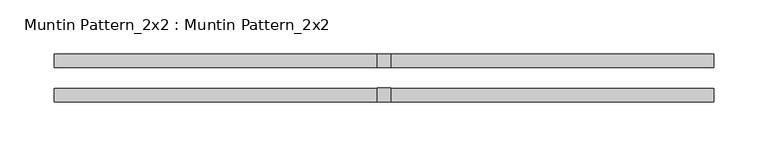
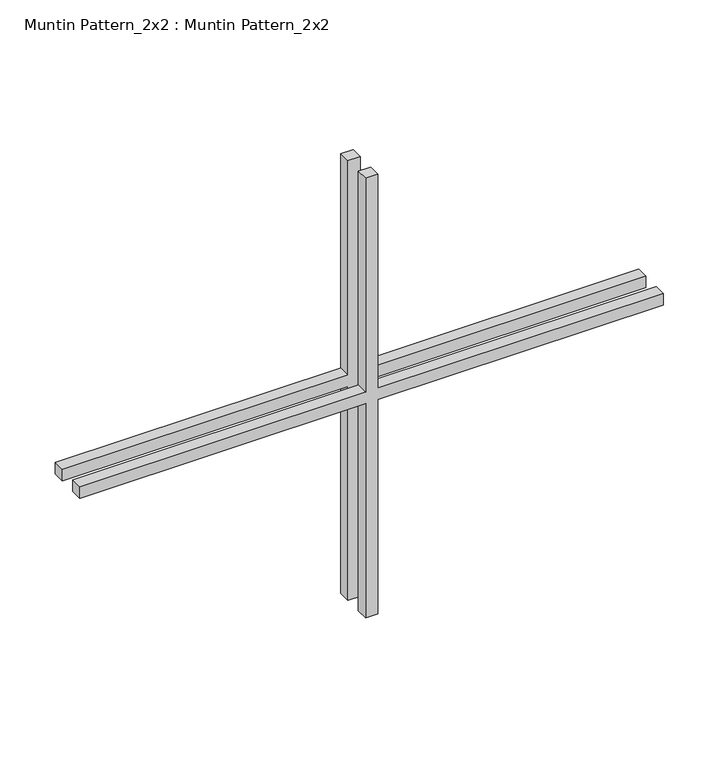
"""IFC4 building model written with IfcOpenShell, lengths in millimetres: proxy geometry, Muntin Pattern_2x2 : Muntin Pattern_2x2."""

from ifc_helpers import new_model, si_unit, frame, origin, place, context, project, spatial, polyline, outline, extrude, source, transform, mapped, element, save


def muntin_pattern_2x2_muntin_pattern_2x2_d064d722(model_context):
    return source(origin(), model_context, "Body", "SweptSolid", [
        extrude(outline(polyline([(249.2375, -6.35), (249.2375, -304.8), (236.5375, -304.8), (236.5375, -6.35), (0.0, -6.35), (0.0, 6.35), (236.5375, 6.35), (236.5375, 304.8), (249.2375, 304.8), (249.2375, 6.35), (485.775, 6.35), (485.775, -6.35), (249.2375, -6.35)])), frame((0.0, -22.225, 0.0), z_axis=(0.0, 1.0, 0.0), x_axis=(0.0, 0.0, 1.0)), (0.0, 0.0, 1.0), 12.7),
        extrude(outline(polyline([(249.2375, -6.35), (249.2375, -304.8), (236.5375, -304.8), (236.5375, -6.35), (0.0, -6.35), (0.0, 6.35), (236.5375, 6.35), (236.5375, 304.8), (249.2375, 304.8), (249.2375, 6.35), (485.775, 6.35), (485.775, -6.35), (249.2375, -6.35)])), frame((0.0, 9.525, 0.0), z_axis=(0.0, 1.0, 0.0), x_axis=(0.0, 0.0, 1.0)), (0.0, 0.0, 1.0), 12.7),
    ])


if __name__ == "__main__":
    model = new_model("IFC4")
    model_context = context("Model", 3, world=origin())
    ifc_project = project(units=[si_unit("LENGTHUNIT", "METRE", prefix="MILLI")], contexts=[model_context])
    site = spatial("IfcSite", under=ifc_project)
    building = spatial("IfcBuilding", under=site)
    placement = place(None, origin())
    muntin_pattern_2x2_muntin_pattern_2x2_shape = muntin_pattern_2x2_muntin_pattern_2x2_d064d722(model_context)
    element("IfcBuildingElementProxy", 1, Name="Muntin Pattern_2x2 : Muntin Pattern_2x2", ObjectType="Muntin Pattern_2x2 : Muntin Pattern_2x2", at=placement, inside=building, context=model_context, shape_type="MappedRepresentation", body=[
        mapped(muntin_pattern_2x2_muntin_pattern_2x2_shape, transform((0.0, 0.0, 0.0), x_axis=(1.0, 0.0, 0.0), y_axis=(0.0, 1.0, 0.0), z_axis=(0.0, 0.0, 1.0))),
    ])
    save(model, "model.ifc")

# Revit data of these elements
# Type "Muntin Pattern_2x2 : Muntin Pattern_2x2"
#   Width [instance default] = 4' - 0"
#   Thickness = 0' - 0 1/2"
#   Height [instance default] = 4' - 0"
#   Distance = 0' - 0 3/4"
#   Interior Material [instance default] = none
#   Exterior Material [instance default] = none
#   Default Elevation = 0
# Element 1 (IfcBuildingElementProxy, "Muntin Pattern_2x2 : Muntin Pattern_2x2")
#   Width = 2' - 0"
#   Height = 1' - 7 1/8"
#   Interior Material = Wood - Stained
#   Exterior Material = Clad - White
#   Materials on its faces: "Clad - White", "Wood - Stained"
# Materials
#   "Clad - White": class "Wood", colour RGB 242 242 238, transparency 0, Cost = 0
#   "Wood - Stained": class "Wood", colour RGB 224 178 126, transparency 0, Cost = 0
